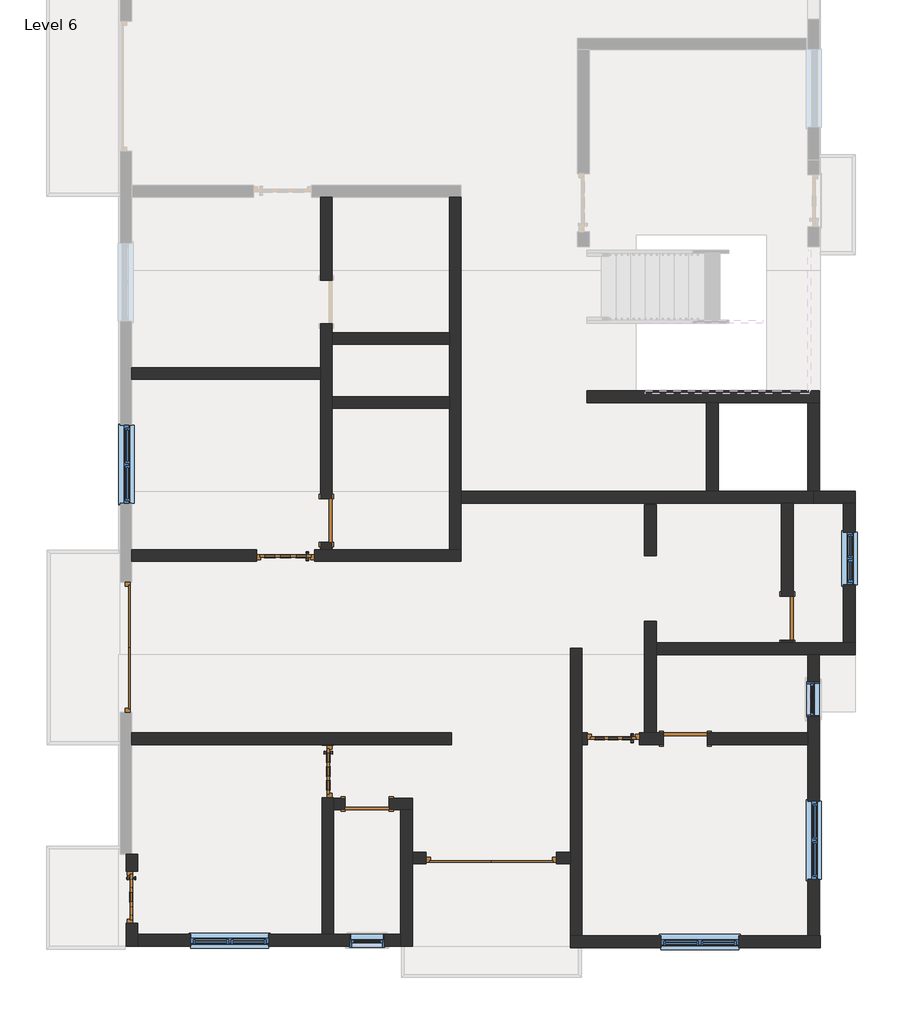
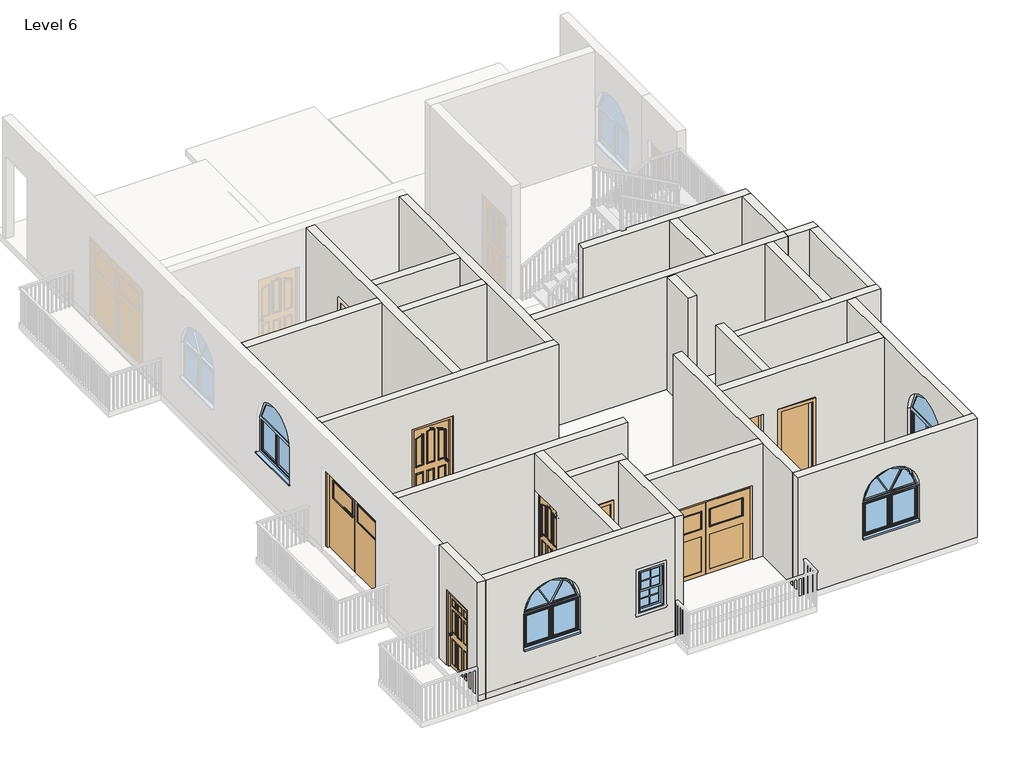
# One storey, part 1 of 7: 27 walls, 10 doors, 7 windows.
"""IFC4 building model written with IfcOpenShell, lengths in millimetres."""

from ifc_helpers import new_model, si_unit, frame, origin, place, context, project, spatial, polyline, circle_curve, outline, extrude, faceted_brep, transform, mapped, element, save
from ifc_brep_helpers import plane_surface, revolved_surface, advanced_brep
from components import doors_extsgl_5_910x2110mm_99758a98, doors_extsgl_6_1010x2110mm_b93c615f, doors_extsgl_6_1010x2110mm_efbaf1af, doors_extsgl_6_910x2110mm_72be2df1, doors_extsgl_6_910x2110mm_b26fcae4, doors_extsgl_6_910x2110mm_5dc58899, doors_extsgl_6_910x2110mm_16d7c084, doors_garage_timber_side_hung_glazing_2270x2050mm_ae99176d, doors_garage_timber_side_hung_glazing_2270x2200mm_badb7014, door_fadea3f2, door_53b1b562, window_679d2811, windows_arched_1360x910mm_c5754810, windows_dbl_w_glazing_bars_910x910mm_41eba874

model = new_model("IFC4")

# Units and contexts
model_context = context("Model", 3, world=origin())
ifc_project = project(units=[si_unit("LENGTHUNIT", "METRE", prefix="MILLI")], contexts=[model_context])

# Site, building, storey
site = spatial("IfcSite", under=ifc_project)
building = spatial("IfcBuilding", under=site)
storey = spatial("IfcBuildingStorey", under=building, Name="Level 6", Elevation=15240.0)

# Doors
placement = place(None, origin())
doors_extsgl_5_910x2110mm_shape = doors_extsgl_5_910x2110mm_99758a98(model_context)
element("IfcDoor", 1, ObjectType="Doors_ExtSgl_5 : 910x2110mm", at=placement, inside=storey, context=model_context, shape_type="MappedRepresentation", body=[
    mapped(doors_extsgl_5_910x2110mm_shape, transform((-6127.6013636, -9759.5108149, 15240.0), x_axis=(0.0, -1.0, 0.0), y_axis=(1.0, 0.0, 0.0), z_axis=(0.0, 0.0, 1.0))),
])
doors_extsgl_6_1010x2110mm_shape = doors_extsgl_6_1010x2110mm_b93c615f(model_context)
doors_extsgl_6_1010x2110mm_2_shape = doors_extsgl_6_1010x2110mm_efbaf1af(model_context)
element("IfcDoor", 2, ObjectType="Doors_ExtSgl_6 : 1010x2110mm", at=placement, inside=storey, context=model_context, shape_type="MappedRepresentation", body=[
    mapped(doors_extsgl_6_1010x2110mm_shape, transform((-3445.8775704, -3805.7037749, 15240.0), x_axis=(-1.0, 0.0, 0.0), y_axis=(0.0, -1.0, 0.0), z_axis=(0.0, 0.0, 1.0))),
    mapped(doors_extsgl_6_1010x2110mm_2_shape, transform((-3445.8775704, -3805.7037749, 15240.0), x_axis=(-1.0, 0.0, 0.0), y_axis=(0.0, -1.0, 0.0), z_axis=(0.0, 0.0, 1.0))),
])
doors_extsgl_6_910x2110mm_shape = doors_extsgl_6_910x2110mm_72be2df1(model_context)
doors_extsgl_6_910x2110mm_2_shape = doors_extsgl_6_910x2110mm_b26fcae4(model_context)
element("IfcDoor", 3, ObjectType="Doors_ExtSgl_6 : 910x2110mm", at=placement, inside=storey, context=model_context, shape_type="MappedRepresentation", body=[
    mapped(doors_extsgl_6_910x2110mm_shape, transform((2269.1224296, -6998.5466225, 15240.0), x_axis=(-1.0, 0.0, 0.0), y_axis=(0.0, -1.0, 0.0), z_axis=(0.0, 0.0, 1.0))),
    mapped(doors_extsgl_6_910x2110mm_2_shape, transform((2269.1224296, -6998.5466225, 15240.0), x_axis=(-1.0, 0.0, 0.0), y_axis=(0.0, -1.0, 0.0), z_axis=(0.0, 0.0, 1.0))),
])
doors_extsgl_6_910x2110mm_3_shape = doors_extsgl_6_910x2110mm_5dc58899(model_context)
doors_extsgl_6_910x2110mm_4_shape = doors_extsgl_6_910x2110mm_16d7c084(model_context)
element("IfcDoor", 4, ObjectType="Doors_ExtSgl_6 : 910x2110mm", at=placement, inside=storey, context=model_context, shape_type="MappedRepresentation", body=[
    mapped(doors_extsgl_6_910x2110mm_3_shape, transform((-2709.3109037, -7568.3747197, 15240.0), x_axis=(0.0, -1.0, 0.0), y_axis=(1.0, 0.0, 0.0), z_axis=(0.0, 0.0, 1.0))),
    mapped(doors_extsgl_6_910x2110mm_4_shape, transform((-2709.3109037, -7568.3747197, 15240.0), x_axis=(0.0, -1.0, 0.0), y_axis=(1.0, 0.0, 0.0), z_axis=(0.0, 0.0, 1.0))),
])
doors_garage_timber_side_hung_glazing_2270x2050mm_shape = doors_garage_timber_side_hung_glazing_2270x2050mm_ae99176d(model_context)
element("IfcDoor", 5, ObjectType="Doors_Garage_Timber_Side_Hung_Glazing : 2270x2050mm", at=placement, inside=storey, context=model_context, shape_type="MappedRepresentation", body=[
    mapped(doors_garage_timber_side_hung_glazing_2270x2050mm_shape, transform((141.8390963, -9078.0694836, 15240.0), x_axis=(-1.0, 0.0, 0.0), y_axis=(0.0, -1.0, 0.0), z_axis=(0.0, 0.0, 1.0))),
])
doors_garage_timber_side_hung_glazing_2270x2200mm_shape = doors_garage_timber_side_hung_glazing_2270x2200mm_badb7014(model_context)
element("IfcDoor", 6, ObjectType="Doors_Garage_Timber_Side_Hung_Glazing : 2270x2200mm", at=placement, inside=storey, context=model_context, shape_type="MappedRepresentation", body=[
    mapped(doors_garage_timber_side_hung_glazing_2270x2200mm_shape, transform((-6229.2013636, -5402.1251987, 15240.0), x_axis=(0.0, 1.0, 0.0), y_axis=(-1.0, 0.0, 0.0), z_axis=(0.0, 0.0, 1.0))),
])
door_shape = door_fadea3f2(model_context)
element("IfcDoor", 7, ObjectType="Single-Flush : 30\" x 80\"", at=placement, inside=storey, context=model_context, shape_type="MappedRepresentation", body=[
    mapped(door_shape, transform((-2023.5109037, -8138.2694836, 15240.0), x_axis=(-1.0, 0.0, 0.0), y_axis=(0.0, -1.0, 0.0), z_axis=(0.0, 0.0, 1.0))),
])
element("IfcDoor", 8, ObjectType="Single-Flush : 30\" x 80\"", at=placement, inside=storey, context=model_context, shape_type="MappedRepresentation", body=[
    mapped(door_shape, transform((5304.3890963, -4897.9037749, 15240.0), x_axis=(0.0, -1.0, 0.0), y_axis=(1.0, 0.0, 0.0), z_axis=(0.0, 0.0, 1.0))),
])
door_2_shape = door_53b1b562(model_context)
element("IfcDoor", 9, ObjectType="Single-Flush : 30\" x 80\"", at=placement, inside=storey, context=model_context, shape_type="MappedRepresentation", body=[
    mapped(door_2_shape, transform((-2734.7109037, -3196.1037749, 15240.0), x_axis=(0.0, 1.0, 0.0), y_axis=(-1.0, 0.0, 0.0), z_axis=(0.0, 0.0, 1.0))),
])
element("IfcDoor", 10, ObjectType="Single-Flush : 30\" x 80\"", at=placement, inside=storey, context=model_context, shape_type="MappedRepresentation", body=[
    mapped(door_2_shape, transform((3526.3890963, -6998.5466225, 15240.0), x_axis=(-1.0, 0.0, 0.0), y_axis=(0.0, -1.0, 0.0), z_axis=(0.0, 0.0, 1.0))),
])

# Walls
element("IfcWall", 11, ObjectType="Generic - 9\" w", at=placement, inside=storey, context=model_context, shape_type="Brep", body=[
    faceted_brep([(6485.4890963, -2688.1037749, 15240.0), (5863.1890963, -2688.1037749, 15240.0), (5761.5890963, -2688.1037749, 15240.0), (5761.5890963, -2688.1037749, 18288.0), (5863.1890963, -2688.1037749, 18288.0), (6485.4890963, -2688.1037749, 18288.0), (6485.4890963, -2891.3037749, 15240.0), (6485.4890963, -2891.3037749, 18288.0), (6282.2890963, -2891.3037749, 18288.0), (5761.5890963, -2891.3037749, 18288.0), (5761.5890963, -2891.3037749, 15240.0), (6282.2890963, -2891.3037749, 15240.0)], [[[0, 1, 2, 3, 4, 5]], [[6, 7, 8, 9, 10, 11]], [[2, 1, 0, 6, 11, 10]], [[3, 2, 10, 9]], [[5, 4, 3, 9, 8, 7]], [[0, 5, 7, 6]]]),
])
element("IfcWall", 12, ObjectType="Generic - 9\" w", at=placement, inside=storey, context=model_context, shape_type="Brep", body=[
    faceted_brep([(5761.5890963, -2688.1037749, 15240.0), (5659.9890963, -2688.1037749, 15240.0), (4097.8890963, -2688.1037749, 15240.0), (3894.6890963, -2688.1037749, 15240.0), (-385.2109037, -2688.1037749, 15240.0), (-385.2109037, -2688.1037749, 18288.0), (3894.6890963, -2688.1037749, 18288.0), (4097.8890963, -2688.1037749, 18288.0), (5659.9890963, -2688.1037749, 18288.0), (5761.5890963, -2688.1037749, 18288.0), (5761.5890963, -2891.3037749, 15240.0), (5761.5890963, -2891.3037749, 18288.0), (5405.9890963, -2891.3037749, 18288.0), (5202.7890963, -2891.3037749, 18288.0), (-385.2109037, -2891.3037749, 18288.0), (-385.2109037, -2891.3037749, 15240.0), (5202.7890963, -2891.3037749, 15240.0), (5405.9890963, -2891.3037749, 15240.0)], [[[0, 1, 2, 3, 4, 5, 6, 7, 8, 9]], [[10, 11, 12, 13, 14, 15, 16, 17]], [[4, 3, 2, 1, 0, 10, 17, 16, 15]], [[9, 8, 7, 6, 5, 14, 13, 12, 11]], [[0, 9, 11, 10]], [[5, 4, 15, 14]]]),
])
element("IfcWall", 13, ObjectType="Generic - 9\" w", at=placement, inside=storey, context=model_context, shape_type="SweptSolid", body=[
    extrude(outline(polyline([(3894.6890963, -2688.1037749), (3894.6890963, -1138.7037749), (4097.8890963, -1138.7037749), (4097.8890963, -2688.1037749), (3894.6890963, -2688.1037749)])), frame((0.0, 0.0, 15240.0), z_axis=(0.0, 0.0, 1.0), x_axis=(1.0, 0.0, 0.0)), (0.0, 0.0, 1.0), 3048.0),
])
element("IfcWall", 14, ObjectType="Generic - 9\" w", at=placement, inside=storey, context=model_context, shape_type="Brep", body=[
    faceted_brep([(5863.1890963, -935.5037749, 15240.0), (1812.4805171, -935.5037749, 15240.0), (1812.4805171, -935.5037749, 18288.0), (5863.1890963, -935.5037749, 18288.0), (5863.1890963, -1138.7037749, 15240.0), (5863.1890963, -1138.7037749, 18288.0), (5659.9890963, -1138.7037749, 18288.0), (4097.8890963, -1138.7037749, 18288.0), (3894.6890963, -1138.7037749, 18288.0), (1812.4805171, -1138.7037749, 18288.0), (1812.4805171, -1138.7037749, 15240.0), (3894.6890963, -1138.7037749, 15240.0), (4097.8890963, -1138.7037749, 15240.0), (5659.9890963, -1138.7037749, 15240.0)], [[[0, 1, 2, 3]], [[4, 5, 6, 7, 8, 9, 10, 11, 12, 13]], [[1, 0, 4, 13, 12, 11, 10]], [[2, 1, 10, 9]], [[3, 2, 9, 8, 7, 6, 5]], [[0, 3, 5, 4]]]),
])
element("IfcWall", 15, ObjectType="Generic - 9\" w", at=placement, inside=storey, context=model_context, shape_type="AdvancedBrep", body=[
    advanced_brep(
    [(1519.7890963, -10638.3037749, 15240.0), (5875.8890963, -10638.3037749, 15240.0), (5875.8890963, -10638.3037749, 18288.0), (1519.7890963, -10638.3037749, 18288.0), (4460.3890963, -10638.3037749, 16154.4), (3100.3890963, -10638.3037749, 16154.4), (3100.3890963, -10638.3037749, 17064.4), (4460.3890963, -10638.3037749, 17064.4), (1519.7890963, -10435.1037749, 15240.0), (1519.7890963, -10435.1037749, 18288.0), (1722.9890963, -10435.1037749, 18288.0), (5659.9890963, -10435.1037749, 18288.0), (5863.1890963, -10435.1037749, 18288.0), (5875.8890963, -10435.1037749, 18288.0), (5875.8890963, -10435.1037749, 15240.0), (5863.1890963, -10435.1037749, 15240.0), (5659.9890963, -10435.1037749, 15240.0), (1722.9890963, -10435.1037749, 15240.0), (4460.3890963, -10435.1037749, 16154.4), (4460.3890963, -10435.1037749, 17064.4), (3100.3890963, -10435.1037749, 17064.4), (3100.3890963, -10435.1037749, 16154.4)],
    [
        (0, 1),
        (1, 2),
        (2, 3),
        (3, 0),
        (4, 5),
        (5, 6),
        (6, 7, circle_curve(frame((3780.3890963, -10638.3037749, 17064.4), z_axis=(0.0, 1.0, 0.0), x_axis=(-1.0, 0.0, 0.0)), 680.0)),
        (7, 4),
        (8, 9),
        (9, 10),
        (10, 11),
        (11, 12),
        (12, 13),
        (13, 14),
        (14, 15),
        (15, 16),
        (16, 17),
        (17, 8),
        (18, 19),
        (19, 20, circle_curve(frame((3780.3890963, -10435.1037749, 17064.4), z_axis=(0.0, -1.0, 0.0), x_axis=(-1.0, 0.0, 0.0)), 680.0)),
        (20, 21),
        (21, 18),
        (0, 8),
        (14, 1),
        (13, 2),
        (9, 3),
        (18, 4),
        (7, 19),
        (6, 20),
        (5, 21),
    ],
    [
        plane_surface(frame((1722.9890963, -10638.3037749, 15240.0), z_axis=(0.0, -1.0, 0.0), x_axis=(1.0, 0.0, 0.0))),
        plane_surface(frame((1722.9890963, -10435.1037749, 15240.0), z_axis=(0.0, 1.0, 0.0), x_axis=(-1.0, 0.0, 0.0))),
        plane_surface(frame((1621.3890963, -10638.3037749, 15240.0), z_axis=(0.0, 0.0, -1.0), x_axis=(0.0, 1.0, 0.0))),
        plane_surface(frame((5875.8890963, -10638.3037749, 15240.0), z_axis=(1.0, 0.0, 0.0), x_axis=(0.0, 1.0, 0.0))),
        plane_surface(frame((5875.8890963, -10638.3037749, 18288.0), z_axis=(0.0, 0.0, 1.0), x_axis=(0.0, 1.0, 0.0))),
        plane_surface(frame((1519.7890963, -5418.6037749, 15240.0), z_axis=(-1.0, 0.0, 0.0), x_axis=(0.0, -1.0, 0.0))),
        plane_surface(frame((4460.3890963, -10435.1037749, 16154.4), z_axis=(-1.0, 0.0, 0.0), x_axis=(0.0, -1.0, 0.0))),
        revolved_surface(polyline([(3100.3890963, -10638.3037749, 17064.4), (3100.3890963, -10435.1037749, 17064.4)]), (3780.3890963, -10435.1037749, 17064.4), (0.0, -1.0, 0.0)),
        plane_surface(frame((3100.3890963, -10435.1037749, 17064.4), z_axis=(1.0, 0.0, 0.0), x_axis=(0.0, -1.0, 0.0))),
        plane_surface(frame((3100.3890963, -10435.1037749, 16154.4), z_axis=(0.0, 0.0, 1.0), x_axis=(0.0, -1.0, 0.0))),
    ],
    [
        (0, [[1, 2, 3, 4], [5, 6, 7, 8]]),
        (1, [[9, 10, 11, 12, 13, 14, 15, 16, 17, 18], [19, 20, 21, 22]]),
        (2, [[-1, 23, -18, -17, -16, -15, 24]]),
        (3, [[-2, -24, -14, 25]]),
        (4, [[-3, -25, -13, -12, -11, -10, 26]]),
        (5, [[-4, -26, -9, -23]]),
        (6, [[-19, 27, -8, 28]]),
        (7, [[-20, -28, -7, 29]]),
        (8, [[-21, -29, -6, 30]]),
        (9, [[-22, -30, -5, -27]]),
    ],
),
])
element("IfcWall", 16, ObjectType="Generic - 9\" w", at=placement, inside=storey, context=model_context, shape_type="AdvancedBrep", body=[
    advanced_brep(
    [(5863.1890963, -10435.1037749, 15240.0), (5863.1890963, -5532.9037749, 15240.0), (5863.1890963, -5532.9037749, 18288.0), (5863.1890963, -10435.1037749, 18288.0), (5863.1890963, -8087.6251987, 16154.4), (5863.1890963, -9447.6251987, 16154.4), (5863.1890963, -9447.6251987, 17064.4), (5863.1890963, -8087.6251987, 17064.4), (5863.1890963, -6618.7537749, 17221.2), (5863.1890963, -6009.1537749, 17221.2), (5863.1890963, -6009.1537749, 16154.4), (5863.1890963, -6618.7537749, 16154.4), (5659.9890963, -10435.1037749, 15240.0), (5659.9890963, -10435.1037749, 18288.0), (5659.9890963, -7100.1466225, 18288.0), (5659.9890963, -6896.9466225, 18288.0), (5659.9890963, -5532.9037749, 18288.0), (5659.9890963, -5532.9037749, 15240.0), (5659.9890963, -6896.9466225, 15240.0), (5659.9890963, -7100.1466225, 15240.0), (5659.9890963, -8087.6251987, 16154.4), (5659.9890963, -8087.6251987, 17064.4), (5659.9890963, -9447.6251987, 17064.4), (5659.9890963, -9447.6251987, 16154.4), (5659.9890963, -6618.7537749, 17221.2), (5659.9890963, -6618.7537749, 16154.4), (5659.9890963, -6009.1537749, 16154.4), (5659.9890963, -6009.1537749, 17221.2)],
    [
        (0, 1),
        (1, 2),
        (2, 3),
        (3, 0),
        (4, 5),
        (5, 6),
        (6, 7, circle_curve(frame((5863.1890963, -8767.6251987, 17064.4), z_axis=(-1.0, 0.0, 0.0), x_axis=(0.0, -1.0, 0.0)), 680.0)),
        (7, 4),
        (8, 9),
        (9, 10),
        (10, 11),
        (11, 8),
        (12, 13),
        (13, 14),
        (14, 15),
        (15, 16),
        (16, 17),
        (17, 18),
        (18, 19),
        (19, 12),
        (20, 21),
        (21, 22, circle_curve(frame((5659.9890963, -8767.6251987, 17064.4), z_axis=(1.0, 0.0, 0.0), x_axis=(0.0, -1.0, 0.0)), 680.0)),
        (22, 23),
        (23, 20),
        (24, 25),
        (25, 26),
        (26, 27),
        (27, 24),
        (0, 12),
        (17, 1),
        (2, 16),
        (13, 3),
        (20, 4),
        (7, 21),
        (6, 22),
        (5, 23),
        (24, 8),
        (11, 25),
        (10, 26),
        (9, 27),
    ],
    [
        plane_surface(frame((5863.1890963, -10435.1037749, 15240.0), z_axis=(1.0, 0.0, 0.0), x_axis=(0.0, 1.0, 0.0))),
        plane_surface(frame((5659.9890963, -10435.1037749, 15240.0), z_axis=(-1.0, 0.0, 0.0), x_axis=(0.0, -1.0, 0.0))),
        plane_surface(frame((5863.1890963, -10536.7037749, 15240.0), z_axis=(0.0, 0.0, -1.0), x_axis=(-1.0, 0.0, 0.0))),
        plane_surface(frame((5863.1890963, -5431.3037749, 18288.0), z_axis=(0.0, 0.0, 1.0), x_axis=(-1.0, 0.0, 0.0))),
        plane_surface(frame((1722.9890963, -10435.1037749, 15240.0), z_axis=(0.0, -1.0, 0.0), x_axis=(-1.0, 0.0, 0.0))),
        plane_surface(frame((3018.3890963, -5532.9037749, 15240.0), z_axis=(0.0, 1.0, 0.0), x_axis=(1.0, 0.0, 0.0))),
        plane_surface(frame((5659.9890963, -8087.6251987, 16154.4), z_axis=(0.0, -1.0, 0.0), x_axis=(1.0, 0.0, 0.0))),
        revolved_surface(polyline([(5863.1890963, -9447.6251987, 17064.4), (5659.9890963, -9447.6251987, 17064.4)]), (5659.9890963, -8767.6251987, 17064.4), (1.0, 0.0, 0.0)),
        plane_surface(frame((5659.9890963, -9447.6251987, 17064.4), z_axis=(0.0, 1.0, 0.0), x_axis=(1.0, 0.0, 0.0))),
        plane_surface(frame((5659.9890963, -9447.6251987, 16154.4), z_axis=(0.0, 0.0, 1.0), x_axis=(1.0, 0.0, 0.0))),
        plane_surface(frame((5659.9890963, -6618.7537749, 17221.2), z_axis=(0.0, 1.0, 0.0), x_axis=(1.0, 0.0, 0.0))),
        plane_surface(frame((5659.9890963, -6618.7537749, 16154.4), z_axis=(0.0, 0.0, 1.0), x_axis=(1.0, 0.0, 0.0))),
        plane_surface(frame((5659.9890963, -6009.1537749, 16154.4), z_axis=(0.0, -1.0, 0.0), x_axis=(1.0, 0.0, 0.0))),
        plane_surface(frame((5659.9890963, -6009.1537749, 17221.2), z_axis=(0.0, 0.0, -1.0), x_axis=(1.0, 0.0, 0.0))),
    ],
    [
        (0, [[1, 2, 3, 4], [5, 6, 7, 8], [9, 10, 11, 12]]),
        (1, [[13, 14, 15, 16, 17, 18, 19, 20], [21, 22, 23, 24], [25, 26, 27, 28]]),
        (2, [[-1, 29, -20, -19, -18, 30]]),
        (3, [[-3, 31, -16, -15, -14, 32]]),
        (4, [[-4, -32, -13, -29]]),
        (5, [[-2, -30, -17, -31]]),
        (6, [[-21, 33, -8, 34]]),
        (7, [[-22, -34, -7, 35]]),
        (8, [[-23, -35, -6, 36]]),
        (9, [[-24, -36, -5, -33]]),
        (10, [[-25, 37, -12, 38]]),
        (11, [[-26, -38, -11, 39]]),
        (12, [[-27, -39, -10, 40]]),
        (13, [[-28, -40, -9, -37]]),
    ],
),
])
element("IfcWall", 17, ObjectType="Generic - 9\" w", at=placement, inside=storey, context=model_context, shape_type="Brep", body=[
    faceted_brep([(5659.9890963, -1138.7037749, 15240.0), (5659.9890963, -2688.1037749, 15240.0), (5659.9890963, -2688.1037749, 18288.0), (5659.9890963, -1138.7037749, 18288.0), (5863.1890963, -1138.7037749, 15240.0), (5863.1890963, -1138.7037749, 18288.0), (5863.1890963, -2688.1037749, 18288.0), (5863.1890963, -2688.1037749, 15240.0), (5761.5890963, -2688.1037749, 15240.0), (5761.5890963, -2688.1037749, 18288.0)], [[[0, 1, 2, 3]], [[4, 5, 6, 7]], [[1, 0, 4, 7, 8]], [[3, 2, 9, 6, 5]], [[2, 1, 8, 7, 6, 9]], [[0, 3, 5, 4]]]),
])
element("IfcWall", 18, ObjectType="Generic - 9\" w", at=placement, inside=storey, context=model_context, shape_type="Brep", body=[
    faceted_brep([(-6229.2013636, -10214.5441482, 17350.0), (-6229.2013636, -10214.5441482, 15240.0), (-6229.2013636, -10612.9037749, 15240.0), (-6229.2013636, -10612.9037749, 18288.0), (-6229.2013636, -9007.7845215, 18288.0), (-6229.2013636, -9007.7845215, 15240.0), (-6229.2013636, -9304.5441482, 15240.0), (-6229.2013636, -9304.5441482, 17350.0), (-6026.0013636, -10612.9037749, 15240.0), (-6026.0013636, -10409.7037749, 15240.0), (-6026.0013636, -10214.5441482, 15240.0), (-6026.0013636, -10214.5441482, 17350.0), (-6026.0013636, -9304.5441482, 17350.0), (-6026.0013636, -9304.5441482, 15240.0), (-6026.0013636, -9007.7845215, 15240.0), (-6026.0013636, -9007.7845215, 18288.0), (-6026.0013636, -10409.7037749, 18288.0), (-6026.0013636, -10612.9037749, 18288.0), (-6127.6013636, -9007.7845215, 15240.0), (-6127.6013636, -9007.7845215, 18288.0)], [[[0, 1, 2, 3, 4, 5, 6, 7]], [[8, 9, 10, 11, 12, 13, 14, 15, 16, 17]], [[6, 5, 18, 14, 13]], [[2, 1, 10, 9, 8]], [[4, 3, 17, 16, 15, 19]], [[5, 4, 19, 15, 14, 18]], [[13, 12, 7, 6]], [[11, 10, 1, 0]], [[12, 11, 0, 7]], [[3, 2, 8, 17]]]),
])
element("IfcWall", 19, ObjectType="Generic - 9\" w", at=placement, inside=storey, context=model_context, shape_type="AdvancedBrep", body=[
    advanced_brep(
    [(-6026.0013636, -10612.9037749, 15240.0), (-1439.3109037, -10612.9037749, 15240.0), (-1439.3109037, -10612.9037749, 18288.0), (-6026.0013636, -10612.9037749, 18288.0), (-3738.4561337, -10612.9037749, 16154.4), (-5098.4561337, -10612.9037749, 16154.4), (-5098.4561337, -10612.9037749, 17064.4), (-3738.4561337, -10612.9037749, 17064.4), (-1718.7109037, -10612.9037749, 17221.2), (-1718.7109037, -10612.9037749, 16154.4), (-2328.3109037, -10612.9037749, 16154.4), (-2328.3109037, -10612.9037749, 17221.2), (-6026.0013636, -10409.7037749, 15240.0), (-6026.0013636, -10409.7037749, 18288.0), (-2810.9109037, -10409.7037749, 18288.0), (-2607.7109037, -10409.7037749, 18288.0), (-1439.3109037, -10409.7037749, 18288.0), (-1439.3109037, -10409.7037749, 15240.0), (-2607.7109037, -10409.7037749, 15240.0), (-2810.9109037, -10409.7037749, 15240.0), (-3738.4561337, -10409.7037749, 16154.4), (-3738.4561337, -10409.7037749, 17064.4), (-5098.4561337, -10409.7037749, 17064.4), (-5098.4561337, -10409.7037749, 16154.4), (-1718.7109037, -10409.7037749, 17221.2), (-2328.3109037, -10409.7037749, 17221.2), (-2328.3109037, -10409.7037749, 16154.4), (-1718.7109037, -10409.7037749, 16154.4)],
    [
        (0, 1),
        (1, 2),
        (2, 3),
        (3, 0),
        (4, 5),
        (5, 6),
        (6, 7, circle_curve(frame((-4418.4561337, -10612.9037749, 17064.4), z_axis=(0.0, 1.0, 0.0), x_axis=(-1.0, 0.0, 0.0)), 680.0)),
        (7, 4),
        (8, 9),
        (9, 10),
        (10, 11),
        (11, 8),
        (12, 13),
        (13, 14),
        (14, 15),
        (15, 16),
        (16, 17),
        (17, 18),
        (18, 19),
        (19, 12),
        (20, 21),
        (21, 22, circle_curve(frame((-4418.4561337, -10409.7037749, 17064.4), z_axis=(0.0, -1.0, 0.0), x_axis=(-1.0, 0.0, 0.0)), 680.0)),
        (22, 23),
        (23, 20),
        (24, 25),
        (25, 26),
        (26, 27),
        (27, 24),
        (0, 12),
        (17, 1),
        (2, 16),
        (13, 3),
        (20, 4),
        (7, 21),
        (6, 22),
        (5, 23),
        (8, 24),
        (27, 9),
        (26, 10),
        (25, 11),
    ],
    [
        plane_surface(frame((-6229.2013636, -10612.9037749, 15240.0), z_axis=(0.0, -1.0, 0.0), x_axis=(1.0, 0.0, 0.0))),
        plane_surface(frame((-6229.2013636, -10409.7037749, 15240.0), z_axis=(0.0, 1.0, 0.0), x_axis=(-1.0, 0.0, 0.0))),
        plane_surface(frame((-6127.6013636, -10612.9037749, 15240.0), z_axis=(0.0, 0.0, -1.0), x_axis=(0.0, 1.0, 0.0))),
        plane_surface(frame((-1337.7109037, -10612.9037749, 18288.0), z_axis=(0.0, 0.0, 1.0), x_axis=(0.0, 1.0, 0.0))),
        plane_surface(frame((-1439.3109037, -8239.8694836, 15240.0), z_axis=(1.0, 0.0, 0.0), x_axis=(0.0, -1.0, 0.0))),
        plane_surface(frame((-6026.0013636, -9109.3845215, 15240.0), z_axis=(-1.0, 0.0, 0.0), x_axis=(0.0, 1.0, 0.0))),
        plane_surface(frame((-3738.4561337, -10409.7037749, 16154.4), z_axis=(-1.0, 0.0, 0.0), x_axis=(0.0, -1.0, 0.0))),
        revolved_surface(polyline([(-5098.4561337, -10612.9037749, 17064.4), (-5098.4561337, -10409.7037749, 17064.4)]), (-4418.4561337, -10409.7037749, 17064.4), (0.0, -1.0, 0.0)),
        plane_surface(frame((-5098.4561337, -10409.7037749, 17064.4), z_axis=(1.0, 0.0, 0.0), x_axis=(0.0, -1.0, 0.0))),
        plane_surface(frame((-5098.4561337, -10409.7037749, 16154.4), z_axis=(0.0, 0.0, 1.0), x_axis=(0.0, -1.0, 0.0))),
        plane_surface(frame((-1718.7109037, -10612.9037749, 17221.2), z_axis=(-1.0, 0.0, 0.0), x_axis=(0.0, 1.0, 0.0))),
        plane_surface(frame((-1718.7109037, -10612.9037749, 16154.4), z_axis=(0.0, 0.0, 1.0), x_axis=(0.0, 1.0, 0.0))),
        plane_surface(frame((-2328.3109037, -10612.9037749, 16154.4), z_axis=(1.0, 0.0, 0.0), x_axis=(0.0, 1.0, 0.0))),
        plane_surface(frame((-2328.3109037, -10612.9037749, 17221.2), z_axis=(0.0, 0.0, -1.0), x_axis=(0.0, 1.0, 0.0))),
    ],
    [
        (0, [[1, 2, 3, 4], [5, 6, 7, 8], [9, 10, 11, 12]]),
        (1, [[13, 14, 15, 16, 17, 18, 19, 20], [21, 22, 23, 24], [25, 26, 27, 28]]),
        (2, [[-1, 29, -20, -19, -18, 30]]),
        (3, [[-3, 31, -16, -15, -14, 32]]),
        (4, [[-2, -30, -17, -31]]),
        (5, [[-4, -32, -13, -29]]),
        (6, [[-21, 33, -8, 34]]),
        (7, [[-22, -34, -7, 35]]),
        (8, [[-23, -35, -6, 36]]),
        (9, [[-24, -36, -5, -33]]),
        (10, [[-9, 37, -28, 38]]),
        (11, [[-10, -38, -27, 39]]),
        (12, [[-11, -39, -26, 40]]),
        (13, [[-12, -40, -25, -37]]),
    ],
),
])
element("IfcWall", 20, ObjectType="Generic -4.5\" p", at=placement, inside=storey, context=model_context, shape_type="Brep", body=[
    faceted_brep([(-2836.3109037, 232.8962251, 15240.0), (-2836.3109037, -529.1037749, 15240.0), (-2836.3109037, -732.3037749, 15240.0), (-2836.3109037, -2815.1037749, 15240.0), (-2836.3109037, -2815.1037749, 17272.0), (-2836.3109037, -3577.1037749, 17272.0), (-2836.3109037, -3577.1037749, 15240.0), (-2836.3109037, -3704.1037749, 15240.0), (-2836.3109037, -3704.1037749, 18288.0), (-2836.3109037, -732.3037749, 18288.0), (-2836.3109037, -529.1037749, 18288.0), (-2836.3109037, 2442.6962251, 18288.0), (-2836.3109037, 2442.6962251, 15240.0), (-2836.3109037, 994.8962251, 15240.0), (-2836.3109037, 994.8962251, 17272.0), (-2836.3109037, 232.8962251, 17272.0), (-2633.1109037, -2815.1037749, 17272.0), (-2633.1109037, -2815.1037749, 15240.0), (-2633.1109037, -1240.3037749, 15240.0), (-2633.1109037, -1037.1037749, 15240.0), (-2633.1109037, -122.7037749, 15240.0), (-2633.1109037, 80.4962251, 15240.0), (-2633.1109037, 232.8962251, 15240.0), (-2633.1109037, 232.8962251, 17272.0), (-2633.1109037, 994.8962251, 17272.0), (-2633.1109037, 994.8962251, 15240.0), (-2633.1109037, 2442.6962251, 15240.0), (-2633.1109037, 2442.6962251, 18288.0), (-2633.1109037, 80.4962251, 18288.0), (-2633.1109037, -122.7037749, 18288.0), (-2633.1109037, -1037.1037749, 18288.0), (-2633.1109037, -1240.3037749, 18288.0), (-2633.1109037, -3704.1037749, 18288.0), (-2633.1109037, -3704.1037749, 15240.0), (-2633.1109037, -3577.1037749, 15240.0), (-2633.1109037, -3577.1037749, 17272.0)], [[[0, 1, 2, 3, 4, 5, 6, 7, 8, 9, 10, 11, 12, 13, 14, 15]], [[16, 17, 18, 19, 20, 21, 22, 23, 24, 25, 26, 27, 28, 29, 30, 31, 32, 33, 34, 35]], [[26, 25, 13, 12]], [[34, 33, 7, 6]], [[22, 21, 20, 19, 18, 17, 3, 2, 1, 0]], [[11, 10, 9, 8, 32, 31, 30, 29, 28, 27]], [[12, 11, 27, 26]], [[8, 7, 33, 32]], [[14, 13, 25, 24]], [[15, 14, 24, 23]], [[0, 15, 23, 22]], [[4, 3, 17, 16]], [[5, 4, 16, 35]], [[6, 5, 35, 34]]]),
])
element("IfcWall", 21, ObjectType="Generic -4.5\" p", at=placement, inside=storey, context=model_context, shape_type="Brep", body=[
    faceted_brep([(-6127.6013636, -3907.3037749, 15240.0), (-3950.9109037, -3907.3037749, 15240.0), (-3950.9109037, -3907.3037749, 17350.0), (-2940.9109037, -3907.3037749, 17350.0), (-2940.9109037, -3907.3037749, 15240.0), (-385.2109037, -3907.3037749, 15240.0), (-385.2109037, -3907.3037749, 18288.0), (-6127.6013636, -3907.3037749, 18288.0), (-3950.9109037, -3704.1037749, 17350.0), (-3950.9109037, -3704.1037749, 15240.0), (-6127.6013636, -3704.1037749, 15240.0), (-6127.6013636, -3704.1037749, 18288.0), (-2836.3109037, -3704.1037749, 18288.0), (-2633.1109037, -3704.1037749, 18288.0), (-588.4109037, -3704.1037749, 18288.0), (-385.2109037, -3704.1037749, 18288.0), (-385.2109037, -3704.1037749, 15240.0), (-588.4109037, -3704.1037749, 15240.0), (-2633.1109037, -3704.1037749, 15240.0), (-2836.3109037, -3704.1037749, 15240.0), (-2940.9109037, -3704.1037749, 15240.0), (-2940.9109037, -3704.1037749, 17350.0)], [[[0, 1, 2, 3, 4, 5, 6, 7]], [[8, 9, 10, 11, 12, 13, 14, 15, 16, 17, 18, 19, 20, 21]], [[10, 9, 1, 0]], [[20, 19, 18, 17, 16, 5, 4]], [[7, 6, 15, 14, 13, 12, 11]], [[6, 5, 16, 15]], [[4, 3, 21, 20]], [[2, 1, 9, 8]], [[3, 2, 8, 21]], [[0, 7, 11, 10]]]),
])
element("IfcWall", 22, ObjectType="Generic -4.5\" p", at=placement, inside=storey, context=model_context, shape_type="Brep", body=[
    faceted_brep([(-385.2109037, -3704.1037749, 15240.0), (-385.2109037, -2891.3037749, 15240.0), (-385.2109037, -2688.1037749, 15240.0), (-385.2109037, 2442.6962251, 15240.0), (-385.2109037, 2442.6962251, 18288.0), (-385.2109037, -2688.1037749, 18288.0), (-385.2109037, -2891.3037749, 18288.0), (-385.2109037, -3704.1037749, 18288.0), (-588.4109037, -3704.1037749, 15240.0), (-588.4109037, -3704.1037749, 18288.0), (-588.4109037, -1240.3037749, 18288.0), (-588.4109037, -1037.1037749, 18288.0), (-588.4109037, -122.7037749, 18288.0), (-588.4109037, 80.4962251, 18288.0), (-588.4109037, 2442.6962251, 18288.0), (-588.4109037, 2442.6962251, 15240.0), (-588.4109037, 80.4962251, 15240.0), (-588.4109037, -122.7037749, 15240.0), (-588.4109037, -1037.1037749, 15240.0), (-588.4109037, -1240.3037749, 15240.0)], [[[0, 1, 2, 3, 4, 5, 6, 7]], [[8, 9, 10, 11, 12, 13, 14, 15, 16, 17, 18, 19]], [[3, 2, 1, 0, 8, 19, 18, 17, 16, 15]], [[7, 6, 5, 4, 14, 13, 12, 11, 10, 9]], [[4, 3, 15, 14]], [[0, 7, 9, 8]]]),
])
element("IfcWall", 23, ObjectType="Generic -4.5\" p", at=placement, inside=storey, context=model_context, shape_type="SweptSolid", body=[
    extrude(outline(polyline([(-588.4109037, -122.7037749), (-2633.1109037, -122.7037749), (-2633.1109037, 80.4962251), (-588.4109037, 80.4962251), (-588.4109037, -122.7037749)])), frame((0.0, 0.0, 15240.0), z_axis=(0.0, 0.0, 1.0), x_axis=(1.0, 0.0, 0.0)), (0.0, 0.0, 1.0), 3048.0),
])
element("IfcWall", 24, ObjectType="Generic -4.5\" p", at=placement, inside=storey, context=model_context, shape_type="SweptSolid", body=[
    extrude(outline(polyline([(-2836.3109037, -732.3037749), (-6127.6013636, -732.3037749), (-6127.6013636, -529.1037749), (-2836.3109037, -529.1037749), (-2836.3109037, -732.3037749)])), frame((0.0, 0.0, 15240.0), z_axis=(0.0, 0.0, 1.0), x_axis=(1.0, 0.0, 0.0)), (0.0, 0.0, 1.0), 3048.0),
])
element("IfcWall", 25, ObjectType="Generic -4.5\" p", at=placement, inside=storey, context=model_context, shape_type="SweptSolid", body=[
    extrude(outline(polyline([(-588.4109037, -1240.3037749), (-2633.1109037, -1240.3037749), (-2633.1109037, -1037.1037749), (-588.4109037, -1037.1037749), (-588.4109037, -1240.3037749)])), frame((0.0, 0.0, 15240.0), z_axis=(0.0, 0.0, 1.0), x_axis=(1.0, 0.0, 0.0)), (0.0, 0.0, 1.0), 3048.0),
])
element("IfcWall", 26, ObjectType="Generic -4.5\" p", at=placement, inside=storey, context=model_context, shape_type="Brep", body=[
    faceted_brep([(-6127.6013636, -7100.1466225, 15240.0), (-2810.9109037, -7100.1466225, 15240.0), (-2607.7109037, -7100.1466225, 15240.0), (-550.3109037, -7100.1466225, 15240.0), (-550.3109037, -7100.1466225, 18288.0), (-2607.7109037, -7100.1466225, 18288.0), (-2810.9109037, -7100.1466225, 18288.0), (-6127.6013636, -7100.1466225, 18288.0), (-6127.6013636, -6896.9466225, 15240.0), (-6127.6013636, -6896.9466225, 18288.0), (-550.3109037, -6896.9466225, 18288.0), (-550.3109037, -6896.9466225, 15240.0)], [[[0, 1, 2, 3, 4, 5, 6, 7]], [[8, 9, 10, 11]], [[3, 2, 1, 0, 8, 11]], [[4, 3, 11, 10]], [[7, 6, 5, 4, 10, 9]], [[0, 7, 9, 8]]]),
])
element("IfcWall", 27, ObjectType="Generic -4.5\" p", at=placement, inside=storey, context=model_context, shape_type="Brep", body=[
    faceted_brep([(-2607.7109037, -10409.7037749, 15240.0), (-2607.7109037, -8239.8694836, 15240.0), (-2607.7109037, -8036.6694836, 15240.0), (-2607.7109037, -8023.4080531, 15240.0), (-2607.7109037, -8023.4080531, 17350.0), (-2607.7109037, -7113.4080531, 17350.0), (-2607.7109037, -7113.4080531, 15240.0), (-2607.7109037, -7100.1466225, 15240.0), (-2607.7109037, -7100.1466225, 18288.0), (-2607.7109037, -8036.6694836, 18288.0), (-2607.7109037, -8239.8694836, 18288.0), (-2607.7109037, -10409.7037749, 18288.0), (-2810.9109037, -8023.4080531, 17350.0), (-2810.9109037, -8023.4080531, 15240.0), (-2810.9109037, -10409.7037749, 15240.0), (-2810.9109037, -10409.7037749, 18288.0), (-2810.9109037, -7100.1466225, 18288.0), (-2810.9109037, -7100.1466225, 15240.0), (-2810.9109037, -7113.4080531, 15240.0), (-2810.9109037, -7113.4080531, 17350.0)], [[[0, 1, 2, 3, 4, 5, 6, 7, 8, 9, 10, 11]], [[12, 13, 14, 15, 16, 17, 18, 19]], [[18, 17, 7, 6]], [[14, 13, 3, 2, 1, 0]], [[11, 10, 9, 8, 16, 15]], [[8, 7, 17, 16]], [[6, 5, 19, 18]], [[4, 3, 13, 12]], [[5, 4, 12, 19]], [[0, 11, 15, 14]]]),
])
element("IfcWall", 28, ObjectType="Generic -4.5\" p", at=placement, inside=storey, context=model_context, shape_type="Brep", body=[
    faceted_brep([(-2607.7109037, -8239.8694836, 15240.0), (-2404.5109037, -8239.8694836, 15240.0), (-2404.5109037, -8239.8694836, 17272.0), (-1642.5109037, -8239.8694836, 17272.0), (-1642.5109037, -8239.8694836, 15240.0), (-1439.3109037, -8239.8694836, 15240.0), (-1236.1109037, -8239.8694836, 15240.0), (-1236.1109037, -8239.8694836, 18288.0), (-1439.3109037, -8239.8694836, 18288.0), (-2607.7109037, -8239.8694836, 18288.0), (-2404.5109037, -8036.6694836, 17272.0), (-2404.5109037, -8036.6694836, 15240.0), (-2607.7109037, -8036.6694836, 15240.0), (-2607.7109037, -8036.6694836, 18288.0), (-1236.1109037, -8036.6694836, 18288.0), (-1236.1109037, -8036.6694836, 15240.0), (-1642.5109037, -8036.6694836, 15240.0), (-1642.5109037, -8036.6694836, 17272.0)], [[[0, 1, 2, 3, 4, 5, 6, 7, 8, 9]], [[10, 11, 12, 13, 14, 15, 16, 17]], [[16, 15, 6, 5, 4]], [[12, 11, 1, 0]], [[9, 8, 7, 14, 13]], [[0, 9, 13, 12]], [[7, 6, 15, 14]], [[2, 1, 11, 10]], [[3, 2, 10, 17]], [[4, 3, 17, 16]]]),
])
element("IfcWall", 29, ObjectType="Generic -4.5\" p", at=placement, inside=storey, context=model_context, shape_type="Brep", body=[
    faceted_brep([(-1439.3109037, -8239.8694836, 15240.0), (-1439.3109037, -10409.7037749, 15240.0), (-1439.3109037, -10612.9037749, 15240.0), (-1439.3109037, -10612.9037749, 18288.0), (-1439.3109037, -10409.7037749, 18288.0), (-1439.3109037, -8239.8694836, 18288.0), (-1236.1109037, -8239.8694836, 15240.0), (-1236.1109037, -8239.8694836, 18288.0), (-1236.1109037, -8976.4694836, 18288.0), (-1236.1109037, -9179.6694836, 18288.0), (-1236.1109037, -10612.9037749, 18288.0), (-1236.1109037, -10612.9037749, 15240.0), (-1236.1109037, -9179.6694836, 15240.0), (-1236.1109037, -8976.4694836, 15240.0)], [[[0, 1, 2, 3, 4, 5]], [[6, 7, 8, 9, 10, 11, 12, 13]], [[2, 1, 0, 6, 13, 12, 11]], [[5, 4, 3, 10, 9, 8, 7]], [[3, 2, 11, 10]], [[0, 5, 7, 6]]]),
])
element("IfcWall", 30, ObjectType="Generic -4.5\" p", at=placement, inside=storey, context=model_context, shape_type="SweptSolid", body=[
    extrude(outline(polyline([(15240.0, -1236.1109037), (15240.0, -993.1609037), (17290.0, -993.1609037), (17290.0, 1276.8390963), (15240.0, 1276.8390963), (15240.0, 1519.7890963), (18288.0, 1519.7890963), (18288.0, -1236.1109037), (15240.0, -1236.1109037)])), frame((0.0, -9179.6694836, 0.0), z_axis=(0.0, 1.0, 0.0), x_axis=(0.0, 0.0, 1.0)), (0.0, 0.0, 1.0), 203.2),
])
element("IfcWall", 31, ObjectType="Generic -4.5\" p", at=placement, inside=storey, context=model_context, shape_type="Brep", body=[
    faceted_brep([(1519.7890963, -5418.6037749, 15240.0), (1519.7890963, -8976.4694836, 15240.0), (1519.7890963, -9179.6694836, 15240.0), (1519.7890963, -10435.1037749, 15240.0), (1519.7890963, -10435.1037749, 18288.0), (1519.7890963, -9179.6694836, 18288.0), (1519.7890963, -8976.4694836, 18288.0), (1519.7890963, -5418.6037749, 18288.0), (1722.9890963, -5418.6037749, 15240.0), (1722.9890963, -5418.6037749, 18288.0), (1722.9890963, -6896.9466225, 18288.0), (1722.9890963, -7100.1466225, 18288.0), (1722.9890963, -10435.1037749, 18288.0), (1722.9890963, -10435.1037749, 15240.0), (1722.9890963, -7100.1466225, 15240.0), (1722.9890963, -6896.9466225, 15240.0)], [[[0, 1, 2, 3, 4, 5, 6, 7]], [[8, 9, 10, 11, 12, 13, 14, 15]], [[3, 2, 1, 0, 8, 15, 14, 13]], [[7, 6, 5, 4, 12, 11, 10, 9]], [[0, 7, 9, 8]], [[4, 3, 13, 12]]]),
])
element("IfcWall", 32, ObjectType="Generic -4.5\" p", at=placement, inside=storey, context=model_context, shape_type="Brep", body=[
    faceted_brep([(2724.0890963, -7100.1466225, 15240.0), (3145.3890963, -7100.1466225, 15240.0), (3145.3890963, -7100.1466225, 17272.0), (3907.3890963, -7100.1466225, 17272.0), (3907.3890963, -7100.1466225, 15240.0), (5659.9890963, -7100.1466225, 15240.0), (5659.9890963, -7100.1466225, 18288.0), (1722.9890963, -7100.1466225, 18288.0), (1722.9890963, -7100.1466225, 15240.0), (1814.0890963, -7100.1466225, 15240.0), (1814.0890963, -7100.1466225, 17350.0), (2724.0890963, -7100.1466225, 17350.0), (3145.3890963, -6896.9466225, 17272.0), (3145.3890963, -6896.9466225, 15240.0), (3018.3890963, -6896.9466225, 15240.0), (2815.1890963, -6896.9466225, 15240.0), (2724.0890963, -6896.9466225, 15240.0), (2724.0890963, -6896.9466225, 17350.0), (1814.0890963, -6896.9466225, 17350.0), (1814.0890963, -6896.9466225, 15240.0), (1722.9890963, -6896.9466225, 15240.0), (1722.9890963, -6896.9466225, 18288.0), (2815.1890963, -6896.9466225, 18288.0), (3018.3890963, -6896.9466225, 18288.0), (5659.9890963, -6896.9466225, 18288.0), (5659.9890963, -6896.9466225, 15240.0), (3907.3890963, -6896.9466225, 15240.0), (3907.3890963, -6896.9466225, 17272.0)], [[[0, 1, 2, 3, 4, 5, 6, 7, 8, 9, 10, 11]], [[12, 13, 14, 15, 16, 17, 18, 19, 20, 21, 22, 23, 24, 25, 26, 27]], [[20, 19, 9, 8]], [[26, 25, 5, 4]], [[16, 15, 14, 13, 1, 0]], [[7, 6, 24, 23, 22, 21]], [[6, 5, 25, 24]], [[8, 7, 21, 20]], [[0, 11, 17, 16]], [[10, 9, 19, 18]], [[11, 10, 18, 17]], [[2, 1, 13, 12]], [[3, 2, 12, 27]], [[4, 3, 27, 26]]]),
])
element("IfcWall", 33, ObjectType="Generic -4.5\" p", at=placement, inside=storey, context=model_context, shape_type="Brep", body=[
    faceted_brep([(3018.3890963, -6896.9466225, 15240.0), (3018.3890963, -5532.9037749, 15240.0), (3018.3890963, -5329.7037749, 15240.0), (3018.3890963, -4949.7445151, 15240.0), (3018.3890963, -4949.7445151, 18288.0), (3018.3890963, -5329.7037749, 18288.0), (3018.3890963, -5532.9037749, 18288.0), (3018.3890963, -6896.9466225, 18288.0), (2815.1890963, -6896.9466225, 15240.0), (2815.1890963, -6896.9466225, 18288.0), (2815.1890963, -4949.7445151, 18288.0), (2815.1890963, -4949.7445151, 15240.0)], [[[0, 1, 2, 3, 4, 5, 6, 7]], [[8, 9, 10, 11]], [[3, 2, 1, 0, 8, 11]], [[4, 3, 11, 10]], [[7, 6, 5, 4, 10, 9]], [[0, 7, 9, 8]]]),
])
element("IfcWall", 34, ObjectType="Generic -4.5\" p", at=placement, inside=storey, context=model_context, shape_type="Brep", body=[
    faceted_brep([(3018.3890963, -5532.9037749, 15240.0), (5659.9890963, -5532.9037749, 15240.0), (5863.1890963, -5532.9037749, 15240.0), (6485.4890963, -5532.9037749, 15240.0), (6485.4890963, -5532.9037749, 18288.0), (5863.1890963, -5532.9037749, 18288.0), (5659.9890963, -5532.9037749, 18288.0), (3018.3890963, -5532.9037749, 18288.0), (3018.3890963, -5329.7037749, 15240.0), (3018.3890963, -5329.7037749, 18288.0), (5202.7890963, -5329.7037749, 18288.0), (5405.9890963, -5329.7037749, 18288.0), (6282.2890963, -5329.7037749, 18288.0), (6485.4890963, -5329.7037749, 18288.0), (6485.4890963, -5329.7037749, 15240.0), (6282.2890963, -5329.7037749, 15240.0), (5405.9890963, -5329.7037749, 15240.0), (5202.7890963, -5329.7037749, 15240.0)], [[[0, 1, 2, 3, 4, 5, 6, 7]], [[8, 9, 10, 11, 12, 13, 14, 15, 16, 17]], [[3, 2, 1, 0, 8, 17, 16, 15, 14]], [[7, 6, 5, 4, 13, 12, 11, 10, 9]], [[0, 7, 9, 8]], [[4, 3, 14, 13]]]),
])
element("IfcWall", 35, ObjectType="Generic -4.5\" p", at=placement, inside=storey, context=model_context, shape_type="SweptSolid", body=[
    extrude(outline(polyline([(-5329.7037749, 15240.0), (-5329.7037749, 18288.0), (-2891.3037749, 18288.0), (-2891.3037749, 15240.0), (-5329.7037749, 15240.0)]), holes=[polyline([(-3401.5037749, 17064.4), (-4311.5037749, 17064.4), (-4311.5037749, 16154.4), (-3401.5037749, 16154.4), (-3401.5037749, 17064.4)])]), frame((6282.2890963, 0.0, 0.0), z_axis=(1.0, 0.0, 0.0), x_axis=(0.0, 1.0, 0.0)), (0.0, 0.0, 1.0), 203.2),
])
element("IfcWall", 36, ObjectType="Generic -4.5\" p", at=placement, inside=storey, context=model_context, shape_type="SweptSolid", body=[
    extrude(outline(polyline([(-5278.9037749, 17272.0), (-5278.9037749, 15240.0), (-5329.7037749, 15240.0), (-5329.7037749, 18288.0), (-2891.3037749, 18288.0), (-2891.3037749, 15240.0), (-4516.9037749, 15240.0), (-4516.9037749, 17272.0), (-5278.9037749, 17272.0)])), frame((5202.7890963, 0.0, 0.0), z_axis=(1.0, 0.0, 0.0), x_axis=(0.0, 1.0, 0.0)), (0.0, 0.0, 1.0), 203.2),
])
element("IfcWall", 37, ObjectType="Generic -4.5\" p", at=placement, inside=storey, context=model_context, shape_type="SweptSolid", body=[
    extrude(outline(polyline([(2815.1890963, -3808.4464026), (2815.1890963, -2916.7037749), (3018.3890963, -2916.7037749), (3018.3890963, -3808.4464026), (2815.1890963, -3808.4464026)])), frame((0.0, 0.0, 15240.0), z_axis=(0.0, 0.0, 1.0), x_axis=(1.0, 0.0, 0.0)), (0.0, 0.0, 1.0), 3048.0),
])

# Windows
window_shape = window_679d2811(model_context)
element("IfcWindow", 38, ObjectType="Window-Double-Hung : 24\" x 42\"", at=placement, inside=storey, context=model_context, shape_type="MappedRepresentation", body=[
    mapped(window_shape, transform((5761.5890963, -6313.9537749, 15240.0), x_axis=(0.0, 1.0, 0.0), y_axis=(-1.0, 0.0, 0.0), z_axis=(0.0, 0.0, 1.0))),
])
element("IfcWindow", 39, ObjectType="Window-Double-Hung : 24\" x 42\"", at=placement, inside=storey, context=model_context, shape_type="MappedRepresentation", body=[
    mapped(window_shape, transform((-2023.5109037, -10511.3037749, 15240.0), x_axis=(-1.0, 0.0, 0.0), y_axis=(0.0, -1.0, 0.0), z_axis=(0.0, 0.0, 1.0))),
])
windows_arched_1360x910mm_shape = windows_arched_1360x910mm_c5754810(model_context)
element("IfcWindow", 40, ObjectType="Windows_Arched : 1360x910mm", at=placement, inside=storey, context=model_context, shape_type="MappedRepresentation", body=[
    mapped(windows_arched_1360x910mm_shape, transform((-6237.6579314, -2503.2037749, 14954.4), x_axis=(0.0, -1.0, 0.0), y_axis=(1.0, 0.0, 0.0), z_axis=(0.0, 0.0, 1.0))),
])
element("IfcWindow", 41, ObjectType="Windows_Arched : 1360x910mm", at=placement, inside=storey, context=model_context, shape_type="MappedRepresentation", body=[
    mapped(windows_arched_1360x910mm_shape, transform((5753.1325284, -9052.6251987, 14954.4), x_axis=(0.0, -1.0, 0.0), y_axis=(1.0, 0.0, 0.0), z_axis=(0.0, 0.0, 1.0))),
])
element("IfcWindow", 42, ObjectType="Windows_Arched : 1360x910mm", at=placement, inside=storey, context=model_context, shape_type="MappedRepresentation", body=[
    mapped(windows_arched_1360x910mm_shape, transform((3495.3890963, -10528.2472071, 14954.4), x_axis=(-1.0, 0.0, 0.0), y_axis=(0.0, -1.0, 0.0), z_axis=(0.0, 0.0, 1.0))),
])
element("IfcWindow", 43, ObjectType="Windows_Arched : 1360x910mm", at=placement, inside=storey, context=model_context, shape_type="MappedRepresentation", body=[
    mapped(windows_arched_1360x910mm_shape, transform((-4703.4561337, -10502.8472071, 14954.4), x_axis=(-1.0, 0.0, 0.0), y_axis=(0.0, -1.0, 0.0), z_axis=(0.0, 0.0, 1.0))),
])
windows_dbl_w_glazing_bars_910x910mm_shape = windows_dbl_w_glazing_bars_910x910mm_41eba874(model_context)
element("IfcWindow", 44, ObjectType="Windows_Dbl_w-Glazing_Bars : 910x910mm", at=placement, inside=storey, context=model_context, shape_type="MappedRepresentation", body=[
    mapped(windows_dbl_w_glazing_bars_910x910mm_shape, transform((6375.4325284, -3986.5037749, 14964.4), x_axis=(0.0, -1.0, 0.0), y_axis=(1.0, 0.0, 0.0), z_axis=(0.0, 0.0, 1.0))),
])

save(model, "model.ifc")

# Revit data of these elements
# Type "Doors_ExtSgl_5 : 910x2110mm"
#   Type Mark = "11"
#   Type Comments = "External Single"
#   Operation = "SingleSwingRight"
#   Construction Type Id = "MDOOR"
#   Keynote = "L20"
#   Analytic Construction = "Metal"
#   Wrap Layers (Int) from Ext = 0' - 6.98819"
#   Wrap Layers (Ext) from Ext = 0' - 4.03543"
#   Thickness = 0' - 1.73228"
#   Stile Top of Lock rail = 3' - 3.37008"
#   Stile Top of Frieze Rail = 5' - 4.96063"
#   Stile Top Rail = 0' - 5.90551"
#   Stile Shutting = 0' - 3.14961"
#   Stile Muntin Rail = 0' - 2.95276"
#   Stile Lock Rail = 0' - 6.88976"
#   Stile Intermediate/Frieze = 0' - 3.14961"
#   Stile Hanging = 0' - 3.14961"
#   Stile Bottom Rail = 0' - 6.88976"
#   Rough Width = 2' - 11.82677"
#   Rough Height = 6' - 11.07087"
#   O/A Frame Width = 0' - 2.51969"
#   Heat Transfer Coefficient (U) = 0.651978 BTU/(h·ft²·°F)
#   Handle Z Distance = 3' - 3.37008"
#   Glazing Thickness = 0' - 0.94488"
#   FrameWidth = 0' - 1.65354"
#   FrameOffset - External = 0' - 0.98425"
#   FrameDepth = 0' - 3.50394"
#   Door Panel Width = 2' - 7.77165"
#   Door Panel Thickness = 0' - 1.73228"
#   Door Panel Height = 6' - 6.74016"
#   DONT CHANGE - Panel Width = 0' - 6.52231"
#   Cill Thickness = 0' - 2.14567"
#   Cill Projection = 0' - 1.1811"
#   Handle X Distance = 0' - 2.95276"
#   Height = 6' - 11.07087"
#   Structural Tolerance = 0' - 0.25591"
#   Tolerance = 0' - 0.11811"
#   Undercut = 0' - 0.15748"
#   Width = 2' - 11.82677"
#   Cill Extension = 0' - 0.98425"
#   Cavity Closer Width = 0' - 1.9685"
#   Cavity Closer Offset from Ext = 0' - 4.03543"
#   Cavity Closer Depth = 0' - 3.34646"
#   Vis - Ironmongery = yes
#   Vis - Cavity Closers = yes
#   Define Thermal Properties by = 1
#   Function = 1
#   Material Glass = Door - Glazing
#   Material Door = Door - Panel
#   Material Frame = Door - Frame/Mullion
#   Material Ironmongery = Door - Handle
#   Visual Light Transmittance = 0
#   Solar Heat Gain Coefficient = 0
#   Wall Closure = (empty or 0)
# Type "Doors_ExtSgl_6 : 1010x2110mm"
#   Type Mark = "12"
#   Type Comments = "External Single"
#   Operation = "SingleSwingRight"
#   Construction Type Id = "SGL"
#   Keynote = "L20"
#   Analytic Construction = "Large single-glazed windows"
#   Wrap Layers (Int) from Ext = 0' - 6.98819"
#   Wrap Layers (Ext) from Ext = 0' - 4.03543"
#   Visual Light Transmittance = 0.9
#   Thickness = 0' - 1.73228"
#   Stile Top of Lock rail = 3' - 3.37008"
#   Stile Top Rail = 0' - 5.90551"
#   Stile Shutting = 0' - 3.54331"
#   Stile Muntin Rail = 0' - 3.54331"
#   Stile Lock Rail = 0' - 6.88976"
#   Stile Hanging = 0' - 3.54331"
#   Stile Bottom Rail = 0' - 6.88976"
#   Solar Heat Gain Coefficient = 0.86
#   Rough Width = 3' - 3.76378"
#   Rough Height = 6' - 11.07087"
#   O/A Frame Width = 0' - 2.51969"
#   Heat Transfer Coefficient (U) = 0.979472 BTU/(h·ft²·°F)
#   Handle Z Distance = 3' - 3.37008"
#   Glazing Thickness = 0' - 0.94488"
#   FrameWidth = 0' - 1.65354"
#   FrameOffset - External = 0' - 0.98425"
#   FrameDepth = 0' - 3.50394"
#   Door Panel Width = 2' - 11.70866"
#   Door Panel Thickness = 0' - 1.73228"
#   Door Panel Height = 6' - 6.74016"
#   DONT CHANGE - Panel Width = 0' - 7.17848"
#   Cill Thickness = 0' - 2.14567"
#   Cill Projection = 0' - 1.1811"
#   Handle X Distance = 0' - 2.95276"
#   Height = 6' - 11.07087"
#   Structural Tolerance = 0' - 0.25591"
#   Tolerance = 0' - 0.11811"
#   Undercut = 0' - 0.15748"
#   Width = 3' - 3.76378"
#   Cill Extension = 0' - 0.98425"
#   Cavity Closer Width = 0' - 1.9685"
#   Cavity Closer Offset from Ext = 0' - 4.03543"
#   Cavity Closer Depth = 0' - 3.34646"
#   Vis - Ironmongery = yes
#   Vis - Cavity Closers = yes
#   Define Thermal Properties by = 1
#   Function = 1
#   Material Glass = Door - Glazing
#   Material Door = Door - Panel
#   Material Frame = Door - Frame/Mullion
#   Material Ironmongery = Door - Handle
#   Wall Closure = (empty or 0)
# Type "Doors_ExtSgl_6 : 910x2110mm"
#   Type Mark = "13"
#   Type Comments = "External Single"
#   Operation = "SingleSwingRight"
#   Construction Type Id = "SGL"
#   Keynote = "L20"
#   Analytic Construction = "Large single-glazed windows"
#   Wrap Layers (Int) from Ext = 0' - 6.98819"
#   Wrap Layers (Ext) from Ext = 0' - 4.03543"
#   Visual Light Transmittance = 0.9
#   Thickness = 0' - 1.73228"
#   Stile Top of Lock rail = 3' - 3.37008"
#   Stile Top Rail = 0' - 5.90551"
#   Stile Shutting = 0' - 3.14961"
#   Stile Muntin Rail = 0' - 2.95276"
#   Stile Lock Rail = 0' - 6.88976"
#   Stile Hanging = 0' - 3.14961"
#   Stile Bottom Rail = 0' - 6.88976"
#   Solar Heat Gain Coefficient = 0.86
#   Rough Width = 2' - 11.82677"
#   Rough Height = 6' - 11.07087"
#   O/A Frame Width = 0' - 2.51969"
#   Heat Transfer Coefficient (U) = 0.979472 BTU/(h·ft²·°F)
#   Handle Z Distance = 3' - 3.37008"
#   Glazing Thickness = 0' - 0.94488"
#   FrameWidth = 0' - 1.65354"
#   FrameOffset - External = 0' - 0.98425"
#   FrameDepth = 0' - 3.50394"
#   Door Panel Width = 2' - 7.77165"
#   Door Panel Thickness = 0' - 1.73228"
#   Door Panel Height = 6' - 6.74016"
#   DONT CHANGE - Panel Width = 0' - 6.52231"
#   Cill Thickness = 0' - 2.14567"
#   Cill Projection = 0' - 1.1811"
#   Handle X Distance = 0' - 2.95276"
#   Height = 6' - 11.07087"
#   Structural Tolerance = 0' - 0.25591"
#   Tolerance = 0' - 0.11811"
#   Undercut = 0' - 0.15748"
#   Width = 2' - 11.82677"
#   Cill Extension = 0' - 0.98425"
#   Cavity Closer Width = 0' - 1.9685"
#   Cavity Closer Offset from Ext = 0' - 4.03543"
#   Cavity Closer Depth = 0' - 3.34646"
#   Vis - Ironmongery = yes
#   Vis - Cavity Closers = yes
#   Define Thermal Properties by = 1
#   Function = 1
#   Material Glass = Door - Glazing
#   Material Door = Door - Panel
#   Material Frame = Door - Frame/Mullion
#   Material Ironmongery = Door - Handle
#   Wall Closure = (empty or 0)
# Type "Doors_Garage_Timber_Side_Hung_Glazing : 2270x2050mm"
#   Type Mark = "8"
#   Type Comments = "External Garage"
#   Operation = "DoubleDoorSingleSwing"
#   Construction Type Id = "GSP4R"
#   Manufacturer = "Revit"
#   Keynote = "L20"
#   Analytic Construction = "1/8 in Pilkington single glazing"
#   Wrap Layers (Ext) from Ext = 0' - 4.03543"
#   Wrap Layers (Int) from Ext = 0' - 6.98819"
#   Visual Light Transmittance = 0.9
#   Thickness = 0' - 1.25984"
#   Stile Top Rail = 0' - 7.87402"
#   Stile Shutting = 0' - 3.93701"
#   Stile Lock Rail = 0' - 7.87402"
#   Stile Hanging = 0' - 6.88976"
#   Stile Bottom Rail = 0' - 9.84252"
#   Solar Heat Gain Coefficient = 0.78
#   Rough Width = 7' - 5.37008"
#   Rough Height = 6' - 8.70866"
#   O/A Frame Width = 0' - 2.51969"
#   Heat Transfer Coefficient (U) = 0.6496 BTU/(h·ft²·°F)
#   Handle Z Distance = 3' - 5.33858"
#   Glazing Panel Height = 1' - 5.71654"
#   FrameWidth = 0' - 1.65354"
#   FrameOffset - External = 0' - 0.98425"
#   FrameDepth = 0' - 3.50394"
#   Door Panel Thickness = 0' - 1.25984"
#   Height = 6' - 8.70866"
#   Structural Tolerance = 0' - 0.31496"
#   Tolerance = 0' - 0.11811"
#   Undercut = 0' - 0.3937"
#   Width = 7' - 5.37008"
#   Cavity Closer Width = 0' - 1.9685"
#   Cavity Closer Offset from Ext = 0' - 4.03543"
#   Cavity Closer Depth = 0' - 3.34646"
#   Vis - Cavity Closers = yes
#   Define Thermal Properties by = 1
#   Function = 1
#   Material Door = Door - Panel
#   Material Frame = Door - Frame/Mullion
#   Material Ironmongery = Door - Handle
#   Wall Closure = (empty or 0)
# Type "Doors_Garage_Timber_Side_Hung_Glazing : 2270x2200mm"
#   Type Mark = "9"
#   Type Comments = "External Garage"
#   Operation = "DoubleDoorSingleSwing"
#   Construction Type Id = "GSP4R"
#   Manufacturer = "Revit"
#   Keynote = "L20"
#   Analytic Construction = "1/8 in Pilkington single glazing"
#   Wrap Layers (Ext) from Ext = 0' - 4.03543"
#   Wrap Layers (Int) from Ext = 0' - 6.98819"
#   Visual Light Transmittance = 0.9
#   Thickness = 0' - 1.25984"
#   Stile Top Rail = 0' - 7.87402"
#   Stile Shutting = 0' - 3.93701"
#   Stile Lock Rail = 0' - 7.87402"
#   Stile Hanging = 0' - 6.88976"
#   Stile Bottom Rail = 0' - 9.84252"
#   Solar Heat Gain Coefficient = 0.78
#   Rough Width = 7' - 5.37008"
#   Rough Height = 7' - 2.61417"
#   O/A Frame Width = 0' - 2.51969"
#   Heat Transfer Coefficient (U) = 0.6496 BTU/(h·ft²·°F)
#   Handle Z Distance = 3' - 5.33858"
#   Glazing Panel Height = 1' - 5.71654"
#   FrameWidth = 0' - 1.65354"
#   FrameOffset - External = 0' - 0.98425"
#   FrameDepth = 0' - 3.50394"
#   Door Panel Thickness = 0' - 1.25984"
#   Height = 7' - 2.61417"
#   Structural Tolerance = 0' - 0.31496"
#   Tolerance = 0' - 0.11811"
#   Undercut = 0' - 0.3937"
#   Width = 7' - 5.37008"
#   Cavity Closer Width = 0' - 1.9685"
#   Cavity Closer Offset from Ext = 0' - 4.03543"
#   Cavity Closer Depth = 0' - 3.34646"
#   Vis - Cavity Closers = yes
#   Define Thermal Properties by = 1
#   Function = 1
#   Material Door = Door - Panel
#   Material Frame = Door - Frame/Mullion
#   Material Ironmongery = Door - Handle
#   Wall Closure = (empty or 0)
# Type "Single-Flush : 30\" x 80\""
#   Type Mark = "5"
